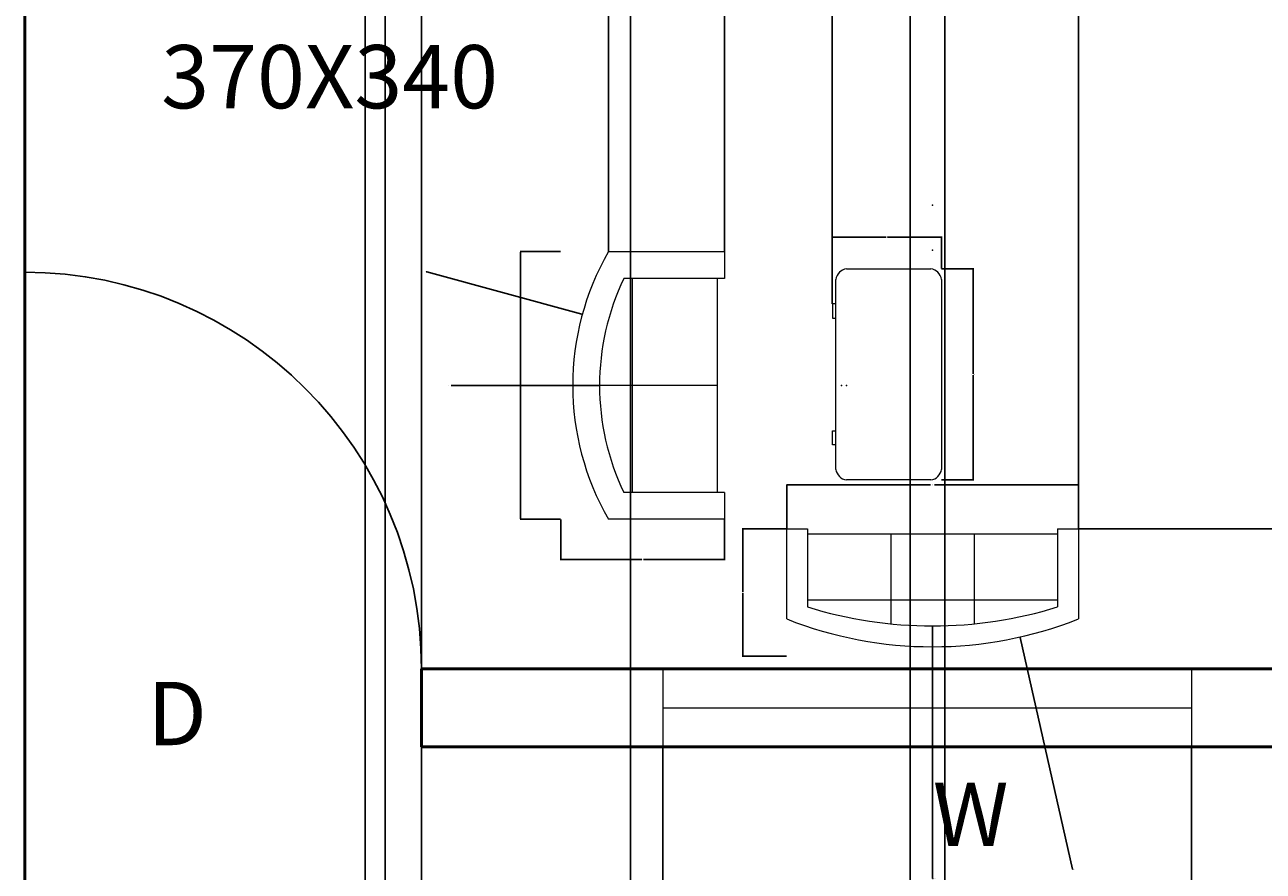
# Model space of a CAD drawing. Units: centimetres. Extents: x 2050 to 3144, y 831 to 2296.
# Tile 3 of 7: x 2553 to 2916, y 1152 to 1401. Entities that reach past the tile are written whole.
import ezdxf

# ---------------------------------------------------------------- set-up
doc = ezdxf.new("R2010")
doc.units = ezdxf.units.CM
for name, color, linetype, lineweight in [('A-ANNO-DIMS', 2, 'Continuous', 18), ('A-ANNO-TEXT', 7, 'Continuous', 18), ('A-AREA-IDEN', 7, 'Continuous', 25), ('A-DOOR', 3, 'Continuous', 25), ('A-FURN', 8, 'Continuous', 18), ('A-GLAZ', 4, 'Continuous', 18), ('A-WALL', 7, 'Continuous', 50)]:
    doc.layers.add(name, color=color, linetype=linetype, lineweight=lineweight)
doc.styles.get("Standard").update_dxf_attribs({"font": 'arial.ttf'})
doc.dimstyles.get("Standard").update_dxf_attribs({"dimtxt": 0.18, "dimasz": 0.18, "dimexe": 0.18, "dimexo": 0.0625, "dimgap": 0.09, "dimtad": 0, "dimtih": 1, "dimtoh": 1, "dimdec": 4, "dimzin": 0, "dimdsep": 46, "dimtxsty": 'Standard', "dimcen": 0.09, "dimadec": 0, "dimazin": 0, "dimtfac": 1, "dimtdec": 4, "dimtofl": 0, "dimtmove": 0, "dimatfit": 3, "dimfxl": 1, "dimtolj": 1, "dimtzin": 0, "dimarcsym": 0})

# ---------------------------------------------------------------- blocks, each defined once
blk = doc.blocks.new('Sofa - Roundback 7 ft.')
for p, q in [((-12.00002, -32.4421), (-12.00003, -6.5971)), ((11.99997, -32.4421), (11.99998, -6.5971)), ((-36.000027, -34), (-36.000027, -11.4696)), ((-35.999844, -13.3819), (35.9998, -13.3819)), ((35.99998, -34), (35.99998, -11.4696)), ((-36.000027, -32.4421), (35.99998, -32.4421))]:
    blk.add_line(p, q)
for points in [[(-36.000027, -34), (-42.000027, -34), (-42.000027, -8)], [(41.99998, -8), (41.99998, -34), (35.99998, -34)]]:
    blk.add_lwpolyline(points)
for centre, radius, start, end in [((0, -114.25), 114.25, 68.43141, 111.5686), ((-0.00001, -127.1968), 121.1968, 72.72033, 107.2797)]:
    blk.add_arc(centre, radius, start, end)
blk = doc.blocks.new('Sofa - Roundback Loveseat 5 ft.')
for p, q in [((0, -32.44198), (0, -5.99998)), ((-24, -33.99998), (-24, -11.46958)), ((-23.9998, -13.38178), (23.99986, -13.38178)), ((24.00004, -33.99998), (24.00004, -11.46958)), ((-24, -32.44198), (24.00004, -32.44198))]:
    blk.add_line(p, q)
for points in [[(-24, -33.99998), (-30, -33.99998), (-30, -7.99998)], [(30.00004, -7.99998), (30.00004, -33.99998), (24.00004, -33.99998)]]:
    blk.add_lwpolyline(points)
for centre, radius, start, end in [((0, -60.24998), 60.24998, 60.13715, 119.8628), ((0, -61.38438), 55.38444, 64.32083, 115.6792)]:
    blk.add_arc(centre, radius, start, end)
blk = doc.blocks.new('Desk - 30 x 60 in.')
for p, q in [((-26.999995, 0), (26.999995, 0)), ((-29.999995, -27), (-29.999995, -3)), ((29.999995, -3), (29.999995, -27)), ((26.999995, -30), (-26.999995, -30)), ((-20.000005, -30), (-20.000005, -31)), ((-20.000005, -31), (-16.000005, -31)), ((-16.000005, -31), (-16.000005, -30)), ((15.999995, -31), (15.999995, -30)), ((19.999995, -31), (15.999995, -31)), ((19.999995, -30), (19.999995, -31))]:
    blk.add_line(p, q)
for centre, start, end in [((-26.499995, -3.5), 98.1301, 171.8699), ((26.499995, -3.5), 8.130102, 81.8699), ((-26.499995, -26.5), 188.1301, 261.8699), ((26.499995, -26.5), 278.1301, 351.8699)]:
    blk.add_arc(centre, 3.535534, start, end)
blk = doc.blocks.new('*D21')
at = {"layer": 'A-ANNO-DIMS', "color": 0, "lineweight": -2, "transparency": 16777216}
for p, q in [((2776.49, 1253.11), (2776.49, 1266.08)), ((2776.67, 1265.9), (2818.72, 1265.9)), ((2861.97, 1265.9), (2819.91, 1265.9)), ((2862.15, 1253.11), (2862.15, 1266.08))]:
    blk.add_line(p, q, dxfattribs=at)
at = {"layer": 'A-ANNO-DIMS', "color": 0, "transparency": 16777216}
for points in [[(2776.67, 1265.93), (2776.67, 1265.87), (2776.49, 1265.9)], [(2861.97, 1265.93), (2861.97, 1265.87), (2862.15, 1265.9)]]:
    blk.add_solid(points, dxfattribs=at)
at = {"layer": 'Defpoints', "color": 0, "transparency": 16777216}
for p in [(2776.49, 1265.9), (2776.49, 1253.05), (2862.15, 1253.05)]:
    blk.add_point(p, dxfattribs=at)
at = {"layer": 'A-ANNO-DIMS', "color": 0, "transparency": 16777216, "insert": (2819.32, 1265.9), "char_height": 0.18, "attachment_point": 5}
blk.add_mtext('\\A1;SOFA 86', dxfattribs=at)
blk = doc.blocks.new('*D22')
at = {"layer": 'A-ANNO-DIMS', "color": 0, "lineweight": -2, "transparency": 16777216}
for p, q in [((2776.43, 1253.05), (2763.46, 1253.05)), ((2763.64, 1252.87), (2763.64, 1234.54)), ((2763.64, 1215.84), (2763.64, 1234.17)), ((2776.43, 1215.66), (2763.46, 1215.66))]:
    blk.add_line(p, q, dxfattribs=at)
at = {"layer": 'A-ANNO-DIMS', "color": 0, "transparency": 16777216}
for points in [[(2763.61, 1252.87), (2763.67, 1252.87), (2763.64, 1253.05)], [(2763.61, 1215.84), (2763.67, 1215.84), (2763.64, 1215.66)]]:
    blk.add_solid(points, dxfattribs=at)
at = {"layer": 'Defpoints', "color": 0, "transparency": 16777216}
for p in [(2776.49, 1253.05), (2763.64, 1215.66), (2776.49, 1215.66)]:
    blk.add_point(p, dxfattribs=at)
at = {"layer": 'A-ANNO-DIMS', "color": 0, "transparency": 16777216, "insert": (2763.64, 1234.36), "char_height": 0.18, "attachment_point": 5}
blk.add_mtext('\\A1;37', dxfattribs=at)
blk = doc.blocks.new('*D23')
at = {"layer": 'A-ANNO-DIMS', "color": 0, "lineweight": -2, "transparency": 16777216}
for p, q in [((2710.09, 1334.43), (2698.18, 1334.43)), ((2698.36, 1334.25), (2698.36, 1295.31)), ((2698.36, 1256), (2698.36, 1294.94)), ((2710.09, 1255.82), (2698.18, 1255.82))]:
    blk.add_line(p, q, dxfattribs=at)
at = {"layer": 'A-ANNO-DIMS', "color": 0, "transparency": 16777216}
for points in [[(2698.33, 1334.25), (2698.39, 1334.25), (2698.36, 1334.43)], [(2698.33, 1256), (2698.39, 1256), (2698.36, 1255.82)]]:
    blk.add_solid(points, dxfattribs=at)
at = {"layer": 'Defpoints', "color": 0, "transparency": 16777216}
for p in [(2698.36, 1334.43), (2710.16, 1334.43), (2710.16, 1255.82)]:
    blk.add_point(p, dxfattribs=at)
at = {"layer": 'A-ANNO-DIMS', "color": 0, "transparency": 16777216, "insert": (2698.36, 1295.12), "char_height": 0.18, "attachment_point": 5}
blk.add_mtext('\\A1;LOVESEAT 79', dxfattribs=at)
blk = doc.blocks.new('*D24')
at = {"layer": 'A-ANNO-DIMS', "color": 0, "lineweight": -2, "transparency": 16777216}
for p, q in [((2710.16, 1255.75), (2710.16, 1243.84)), ((2758.2, 1255.75), (2758.2, 1243.84)), ((2710.34, 1244.02), (2733.95, 1244.02)), ((2758.02, 1244.02), (2734.4, 1244.02))]:
    blk.add_line(p, q, dxfattribs=at)
at = {"layer": 'A-ANNO-DIMS', "color": 0, "transparency": 16777216}
for points in [[(2710.34, 1244.05), (2710.34, 1243.99), (2710.16, 1244.02)], [(2758.02, 1244.05), (2758.02, 1243.99), (2758.2, 1244.02)]]:
    blk.add_solid(points, dxfattribs=at)
at = {"layer": 'Defpoints', "color": 0, "transparency": 16777216}
for p in [(2710.16, 1255.82), (2758.2, 1255.82), (2710.16, 1244.02)]:
    blk.add_point(p, dxfattribs=at)
at = {"layer": 'A-ANNO-DIMS', "color": 0, "transparency": 16777216, "insert": (2734.18, 1244.02), "char_height": 0.18, "attachment_point": 5}
blk.add_mtext('\\A1;48', dxfattribs=at)
blk = doc.blocks.new('*D29')
at = {"layer": 'A-ANNO-DIMS', "color": 0, "lineweight": -2, "transparency": 16777216}
for p, q in [((2822, 1329.39), (2831.42, 1329.39)), ((2831.24, 1329.21), (2831.24, 1298.57)), ((2831.24, 1267.55), (2831.24, 1298.2)), ((2822, 1267.37), (2831.42, 1267.37))]:
    blk.add_line(p, q, dxfattribs=at)
at = {"layer": 'A-ANNO-DIMS', "color": 0, "transparency": 16777216}
for points in [[(2831.21, 1329.21), (2831.27, 1329.21), (2831.24, 1329.39)], [(2831.21, 1267.55), (2831.27, 1267.55), (2831.24, 1267.37)]]:
    blk.add_solid(points, dxfattribs=at)
at = {"layer": 'Defpoints', "color": 0, "transparency": 16777216}
for p in [(2821.94, 1329.39), (2821.94, 1267.37), (2831.24, 1267.37)]:
    blk.add_point(p, dxfattribs=at)
at = {"layer": 'A-ANNO-DIMS', "color": 0, "transparency": 16777216, "insert": (2831.24, 1298.38), "char_height": 0.18, "attachment_point": 5}
blk.add_mtext('\\A1;DESK 62', dxfattribs=at)
blk = doc.blocks.new('*D30')
at = {"layer": 'A-ANNO-DIMS', "color": 0, "lineweight": -2, "transparency": 16777216}
for p, q in [((2789.89, 1329.46), (2789.89, 1338.88)), ((2790.07, 1338.7), (2805.7, 1338.7)), ((2821.76, 1338.7), (2806.14, 1338.7)), ((2821.94, 1329.46), (2821.94, 1338.88))]:
    blk.add_line(p, q, dxfattribs=at)
at = {"layer": 'A-ANNO-DIMS', "color": 0, "transparency": 16777216}
for points in [[(2790.07, 1338.73), (2790.07, 1338.67), (2789.89, 1338.7)], [(2821.76, 1338.73), (2821.76, 1338.67), (2821.94, 1338.7)]]:
    blk.add_solid(points, dxfattribs=at)
at = {"layer": 'Defpoints', "color": 0, "transparency": 16777216}
for p in [(2821.94, 1338.7), (2789.89, 1329.39), (2821.94, 1329.39)]:
    blk.add_point(p, dxfattribs=at)
at = {"layer": 'A-ANNO-DIMS', "color": 0, "transparency": 16777216, "insert": (2805.92, 1338.7), "char_height": 0.18, "attachment_point": 5}
blk.add_mtext('\\A1;32', dxfattribs=at)
blk = doc.blocks.new('*D48')
at = {"layer": 'A-ANNO-DIMS', "color": 0, "lineweight": -2, "transparency": 16777216}
for p, q in [((2552.73, 1211.94), (2552.73, 2154.53)), ((2552.91, 2154.35), (2610.59, 2154.35)), ((2669.05, 2154.35), (2611.37, 2154.35)), ((2669.23, 1211.94), (2669.23, 2154.53))]:
    blk.add_line(p, q, dxfattribs=at)
at = {"layer": 'A-ANNO-DIMS', "color": 0, "transparency": 16777216}
for points in [[(2552.91, 2154.38), (2552.91, 2154.32), (2552.73, 2154.35)], [(2669.05, 2154.38), (2669.05, 2154.32), (2669.23, 2154.35)]]:
    blk.add_solid(points, dxfattribs=at)
at = {"layer": 'Defpoints', "color": 0, "transparency": 16777216}
for p in [(2669.23, 2154.35), (2552.73, 1211.87), (2669.23, 1211.87)]:
    blk.add_point(p, dxfattribs=at)
at = {"layer": 'A-ANNO-DIMS', "color": 0, "transparency": 16777216, "insert": (2610.98, 2154.35), "char_height": 0.18, "attachment_point": 5}
blk.add_mtext('\\A1;116.5', dxfattribs=at)
blk = doc.blocks.new('*D49')
at = {"layer": 'A-ANNO-DIMS', "color": 0, "lineweight": -2, "transparency": 16777216}
for p, q in [((2669.23, 1188.95), (2669.23, 1009.53)), ((2740.09, 1188.95), (2740.09, 1009.53)), ((2669.41, 1009.71), (2704.27, 1009.71)), ((2739.91, 1009.71), (2705.05, 1009.71))]:
    blk.add_line(p, q, dxfattribs=at)
at = {"layer": 'A-ANNO-DIMS', "color": 0, "transparency": 16777216}
for points in [[(2669.41, 1009.74), (2669.41, 1009.68), (2669.23, 1009.71)], [(2739.91, 1009.74), (2739.91, 1009.68), (2740.09, 1009.71)]]:
    blk.add_solid(points, dxfattribs=at)
at = {"layer": 'Defpoints', "color": 0, "transparency": 16777216}
for p in [(2669.23, 1189.01), (2740.09, 1189.01), (2740.09, 1009.71)]:
    blk.add_point(p, dxfattribs=at)
at = {"layer": 'A-ANNO-DIMS', "color": 0, "transparency": 16777216, "insert": (2704.66, 1009.71), "char_height": 0.18, "attachment_point": 5}
blk.add_mtext('\\A1;70.86', dxfattribs=at)
blk = doc.blocks.new('*D50')
at = {"layer": 'A-ANNO-DIMS', "color": 0, "lineweight": -2, "transparency": 16777216}
for p, q in [((2740.09, 1188.95), (2740.09, 1009.53)), ((2895.36, 1188.95), (2895.36, 1009.53)), ((2740.27, 1009.71), (2817.27, 1009.71)), ((2895.18, 1009.71), (2818.18, 1009.71))]:
    blk.add_line(p, q, dxfattribs=at)
at = {"layer": 'A-ANNO-DIMS', "color": 0, "transparency": 16777216}
for points in [[(2740.27, 1009.74), (2740.27, 1009.68), (2740.09, 1009.71)], [(2895.18, 1009.74), (2895.18, 1009.68), (2895.36, 1009.71)]]:
    blk.add_solid(points, dxfattribs=at)
at = {"layer": 'Defpoints', "color": 0, "transparency": 16777216}
for p in [(2740.09, 1189.01), (2895.36, 1189.01), (2895.36, 1009.71)]:
    blk.add_point(p, dxfattribs=at)
at = {"layer": 'A-ANNO-DIMS', "color": 0, "transparency": 16777216, "insert": (2817.72, 1009.71), "char_height": 0.18, "attachment_point": 5}
blk.add_mtext('\\A1;155.27', dxfattribs=at)
blk = doc.blocks.new('*D59')
at = {"layer": 'A-ANNO-DIMS', "color": 0, "lineweight": -2, "transparency": 16777216}
for p, q in [((2862.15, 1253.11), (2862.15, 2154.53)), ((2862.33, 2154.35), (2907.04, 2154.35)), ((2952.55, 2154.35), (2907.83, 2154.35)), ((2952.73, 1211.94), (2952.73, 2154.53))]:
    blk.add_line(p, q, dxfattribs=at)
at = {"layer": 'A-ANNO-DIMS', "color": 0, "transparency": 16777216}
for points in [[(2862.33, 2154.38), (2862.33, 2154.32), (2862.15, 2154.35)], [(2952.55, 2154.38), (2952.55, 2154.32), (2952.73, 2154.35)]]:
    blk.add_solid(points, dxfattribs=at)
at = {"layer": 'Defpoints', "color": 0, "transparency": 16777216}
for p in [(2952.73, 2154.35), (2862.15, 1253.05), (2952.73, 1211.87)]:
    blk.add_point(p, dxfattribs=at)
at = {"layer": 'A-ANNO-DIMS', "color": 0, "transparency": 16777216, "insert": (2907.44, 2154.35), "char_height": 0.18, "attachment_point": 5}
blk.add_mtext('\\A1;90.58', dxfattribs=at)
blk = doc.blocks.new('*D60')
at = {"layer": 'A-ANNO-DIMS', "color": 0, "lineweight": -2, "transparency": 16777216}
for p, q in [((2862.21, 1253.05), (3042.37, 1253.05)), ((3042.19, 1252.87), (3042.19, 1232.65)), ((3042.19, 1212.05), (3042.19, 1232.28)), ((2895.42, 1211.87), (3042.37, 1211.87))]:
    blk.add_line(p, q, dxfattribs=at)
at = {"layer": 'A-ANNO-DIMS', "color": 0, "transparency": 16777216}
for points in [[(3042.16, 1252.87), (3042.22, 1252.87), (3042.19, 1253.05)], [(3042.16, 1212.05), (3042.22, 1212.05), (3042.19, 1211.87)]]:
    blk.add_solid(points, dxfattribs=at)
at = {"layer": 'Defpoints', "color": 0, "transparency": 16777216}
for p in [(2862.15, 1253.05), (2895.36, 1211.87), (3042.19, 1211.87)]:
    blk.add_point(p, dxfattribs=at)
at = {"layer": 'A-ANNO-DIMS', "color": 0, "transparency": 16777216, "insert": (3042.19, 1232.46), "char_height": 0.18, "attachment_point": 5}
blk.add_mtext('\\A1;41.18', dxfattribs=at)
blk = doc.blocks.new('*D61')
at = {"layer": 'A-ANNO-DIMS', "color": 0, "lineweight": -2, "transparency": 16777216}
for p, q in [((2552.73, 1328.44), (2552.73, 2154.53)), ((2552.91, 2154.35), (2638.04, 2154.35)), ((2723.95, 2154.35), (2638.81, 2154.35)), ((2724.13, 1334.5), (2724.13, 2154.53))]:
    blk.add_line(p, q, dxfattribs=at)
at = {"layer": 'A-ANNO-DIMS', "color": 0, "transparency": 16777216}
for points in [[(2552.91, 2154.38), (2552.91, 2154.32), (2552.73, 2154.35)], [(2723.95, 2154.38), (2723.95, 2154.32), (2724.13, 2154.35)]]:
    blk.add_solid(points, dxfattribs=at)
at = {"layer": 'Defpoints', "color": 0, "transparency": 16777216}
for p in [(2724.13, 2154.35), (2724.13, 1334.43), (2552.73, 1328.38)]:
    blk.add_point(p, dxfattribs=at)
at = {"layer": 'A-ANNO-DIMS', "color": 0, "transparency": 16777216, "insert": (2638.43, 2154.35), "char_height": 0.18, "attachment_point": 5}
blk.add_mtext('\\A1;171.4', dxfattribs=at)
blk = doc.blocks.new('*D62')
at = {"layer": 'A-ANNO-DIMS', "color": 0, "lineweight": -2, "transparency": 16777216}
for p, q in [((2758.2, 1334.5), (2758.2, 2154.53)), ((2758.38, 2154.35), (2773.58, 2154.35)), ((2789.71, 2154.35), (2774.51, 2154.35)), ((2789.89, 1319.12), (2789.89, 2154.53))]:
    blk.add_line(p, q, dxfattribs=at)
at = {"layer": 'A-ANNO-DIMS', "color": 0, "transparency": 16777216}
for points in [[(2758.38, 2154.38), (2758.38, 2154.32), (2758.2, 2154.35)], [(2789.71, 2154.38), (2789.71, 2154.32), (2789.89, 2154.35)]]:
    blk.add_solid(points, dxfattribs=at)
at = {"layer": 'Defpoints', "color": 0, "transparency": 16777216}
for p in [(2789.89, 2154.35), (2758.2, 1334.43), (2789.89, 1319.06)]:
    blk.add_point(p, dxfattribs=at)
at = {"layer": 'A-ANNO-DIMS', "color": 0, "transparency": 16777216, "insert": (2774.05, 2154.35), "char_height": 0.18, "attachment_point": 5}
blk.add_mtext('\\A1;31.696', dxfattribs=at)
blk = doc.blocks.new('*D65')
at = {"layer": 'A-ANNO-DIMS', "color": 0, "lineweight": -2, "transparency": 16777216}
for p, q in [((2812.73, 1924.83), (2812.73, 1009.53)), ((2822.89, 1914.67), (2822.89, 1009.53)), ((2812.91, 1009.71), (2817.42, 1009.71)), ((2822.71, 1009.71), (2818.19, 1009.71))]:
    blk.add_line(p, q, dxfattribs=at)
at = {"layer": 'A-ANNO-DIMS', "color": 0, "transparency": 16777216}
for points in [[(2812.91, 1009.74), (2812.91, 1009.68), (2812.73, 1009.71)], [(2822.71, 1009.74), (2822.71, 1009.68), (2822.89, 1009.71)]]:
    blk.add_solid(points, dxfattribs=at)
at = {"layer": 'Defpoints', "color": 0, "transparency": 16777216}
for p in [(2812.73, 1924.89), (2822.89, 1914.73), (2822.89, 1009.71)]:
    blk.add_point(p, dxfattribs=at)
at = {"layer": 'A-ANNO-DIMS', "color": 0, "transparency": 16777216, "insert": (2817.81, 1009.71), "char_height": 0.18, "attachment_point": 5}
blk.add_mtext('\\A1;10.16', dxfattribs=at)
blk = doc.blocks.new('*D68')
at = {"layer": 'A-ANNO-DIMS', "color": 0, "lineweight": -2, "transparency": 16777216}
for p, q in [((2652.73, 1914.67), (2652.73, 1009.53)), ((2730.58, 1841.3), (2730.58, 1009.53)), ((2652.91, 1009.71), (2691.26, 1009.71)), ((2730.4, 1009.71), (2692.05, 1009.71))]:
    blk.add_line(p, q, dxfattribs=at)
at = {"layer": 'A-ANNO-DIMS', "color": 0, "transparency": 16777216}
for points in [[(2652.91, 1009.74), (2652.91, 1009.68), (2652.73, 1009.71)], [(2730.4, 1009.74), (2730.4, 1009.68), (2730.58, 1009.71)]]:
    blk.add_solid(points, dxfattribs=at)
at = {"layer": 'Defpoints', "color": 0, "transparency": 16777216}
for p in [(2652.73, 1914.73), (2730.58, 1841.36), (2730.58, 1009.71)]:
    blk.add_point(p, dxfattribs=at)
at = {"layer": 'A-ANNO-DIMS', "color": 0, "transparency": 16777216, "insert": (2691.65, 1009.71), "char_height": 0.18, "attachment_point": 5}
blk.add_mtext('\\A1;77.85', dxfattribs=at)
blk = doc.blocks.new('*D73')
at = {"layer": 'A-ANNO-DIMS', "color": 0, "lineweight": -2, "transparency": 16777216}
for p, q in [((2658.57, 1971.45), (2658.57, 1009.53)), ((2652.73, 1924.83), (2652.73, 1009.53)), ((2652.91, 1009.71), (2655.26, 1009.71)), ((2658.39, 1009.71), (2656.04, 1009.71))]:
    blk.add_line(p, q, dxfattribs=at)
at = {"layer": 'A-ANNO-DIMS', "color": 0, "transparency": 16777216}
for points in [[(2652.91, 1009.74), (2652.91, 1009.68), (2652.73, 1009.71)], [(2658.39, 1009.74), (2658.39, 1009.68), (2658.57, 1009.71)]]:
    blk.add_solid(points, dxfattribs=at)
at = {"layer": 'Defpoints', "color": 0, "transparency": 16777216}
for p in [(2658.57, 1971.51), (2652.73, 1924.89), (2658.57, 1009.71)]:
    blk.add_point(p, dxfattribs=at)
at = {"layer": 'A-ANNO-DIMS', "color": 0, "transparency": 16777216, "insert": (2655.65, 1009.71), "char_height": 0.18, "attachment_point": 5}
blk.add_mtext('\\A1;5.847', dxfattribs=at)
blk = doc.blocks.new('*D74')
at = {"layer": 'A-ANNO-DIMS', "color": 0, "lineweight": -2, "transparency": 16777216}
for p, q in [((2952.73, 2064.83), (2952.73, 1009.53)), ((2822.89, 2004.16), (2822.89, 1009.53)), ((2823.07, 1009.71), (2887.35, 1009.71)), ((2952.55, 1009.71), (2888.26, 1009.71))]:
    blk.add_line(p, q, dxfattribs=at)
at = {"layer": 'A-ANNO-DIMS', "color": 0, "transparency": 16777216}
for points in [[(2823.07, 1009.74), (2823.07, 1009.68), (2822.89, 1009.71)], [(2952.55, 1009.74), (2952.55, 1009.68), (2952.73, 1009.71)]]:
    blk.add_solid(points, dxfattribs=at)
at = {"layer": 'Defpoints', "color": 0, "transparency": 16777216}
for p in [(2952.73, 2064.89), (2822.89, 2004.22), (2952.73, 1009.71)]:
    blk.add_point(p, dxfattribs=at)
at = {"layer": 'A-ANNO-DIMS', "color": 0, "transparency": 16777216, "insert": (2887.81, 1009.71), "char_height": 0.18, "attachment_point": 5}
blk.add_mtext('\\A1;129.84', dxfattribs=at)
blk = doc.blocks.new('*D77')
at = {"layer": 'A-ANNO-DIMS', "color": 0, "lineweight": -2, "transparency": 16777216}
for p, q in [((2819.23, 1348.09), (2819.41, 1348.09)), ((2819.32, 1348), (2819.32, 1348.18)), ((2819.32, 1150.35), (2819.32, 1224.32)), ((2819.5, 1150.35), (2819.32, 1150.35))]:
    blk.add_line(p, q, dxfattribs=at)
at = {"layer": 'A-ANNO-DIMS', "color": 0, "transparency": 16777216}
blk.add_solid([(2819.35, 1224.32), (2819.29, 1224.32), (2819.32, 1224.5)], dxfattribs=at)
at = {"layer": 'Defpoints', "color": 0, "transparency": 16777216}
for p in [(2819.32, 1348.09), (2819.32, 1224.5)]:
    blk.add_point(p, dxfattribs=at)
at = {"layer": 'A-ANNO-DIMS', "color": 0, "transparency": 16777216, "insert": (2820.05, 1150.35), "char_height": 0.18, "attachment_point": 5}
blk.add_mtext('\\A1;R123.59', dxfattribs=at)
blk = doc.blocks.new('*D78')
at = {"layer": 'A-ANNO-DIMS', "color": 0, "lineweight": -2, "transparency": 16777216}
for p, q in [((2819.23, 1334.88), (2819.41, 1334.88)), ((2819.32, 1334.79), (2819.32, 1334.97)), ((2860.41, 1153.07), (2845.04, 1221.07)), ((2860.59, 1153.07), (2860.41, 1153.07))]:
    blk.add_line(p, q, dxfattribs=at)
at = {"layer": 'A-ANNO-DIMS', "color": 0, "transparency": 16777216}
blk.add_solid([(2845.07, 1221.08), (2845.01, 1221.07), (2845, 1221.25)], dxfattribs=at)
at = {"layer": 'Defpoints', "color": 0, "transparency": 16777216}
for p in [(2819.32, 1334.88), (2845, 1221.25)]:
    blk.add_point(p, dxfattribs=at)
at = {"layer": 'A-ANNO-DIMS', "color": 0, "transparency": 16777216, "insert": (2861.07, 1153.07), "char_height": 0.18, "attachment_point": 5}
blk.add_mtext('\\A1;R116.5', dxfattribs=at)
blk = doc.blocks.new('*D79')
at = {"layer": 'A-ANNO-DIMS', "color": 0, "lineweight": -2, "transparency": 16777216}
for p, q in [((2670.6, 1328.54), (2670.78, 1328.54)), ((2670.78, 1328.54), (2716.29, 1316.06)), ((2792.5, 1295.12), (2792.68, 1295.12)), ((2792.59, 1295.03), (2792.59, 1295.21))]:
    blk.add_line(p, q, dxfattribs=at)
at = {"layer": 'A-ANNO-DIMS', "color": 0, "transparency": 16777216}
blk.add_solid([(2716.3, 1316.09), (2716.28, 1316.03), (2716.46, 1316.01)], dxfattribs=at)
at = {"layer": 'Defpoints', "color": 0, "transparency": 16777216}
for p in [(2716.46, 1316.01), (2792.59, 1295.12)]:
    blk.add_point(p, dxfattribs=at)
at = {"layer": 'A-ANNO-DIMS', "color": 0, "transparency": 16777216, "insert": (2670.12, 1328.54), "char_height": 0.18, "attachment_point": 5}
blk.add_mtext('\\A1;R78.94', dxfattribs=at)
blk = doc.blocks.new('*D80')
at = {"layer": 'A-ANNO-DIMS', "color": 0, "lineweight": -2, "transparency": 16777216}
for p, q in [((2677.97, 1295.12), (2721.33, 1295.12)), ((2793.99, 1295.12), (2794.17, 1295.12)), ((2794.08, 1295.03), (2794.08, 1295.21))]:
    blk.add_line(p, q, dxfattribs=at)
at = {"layer": 'A-ANNO-DIMS', "color": 0, "transparency": 16777216}
blk.add_solid([(2721.33, 1295.16), (2721.33, 1295.1), (2721.51, 1295.12)], dxfattribs=at)
at = {"layer": 'Defpoints', "color": 0, "transparency": 16777216}
for p in [(2721.51, 1295.12), (2794.08, 1295.12)]:
    blk.add_point(p, dxfattribs=at)
at = {"layer": 'A-ANNO-DIMS', "color": 0, "transparency": 16777216, "insert": (2677.49, 1295.12), "char_height": 0.18, "attachment_point": 5}
blk.add_mtext('\\A1;R72.57', dxfattribs=at)

msp = doc.modelspace()

# ---------------------------------------------------------------- linework, layer by layer
at = {"layer": 'A-DOOR'}
msp.add_line((2552.7265, 1211.8748), (2552.7265, 1338.3548), dxfattribs=at)
msp.add_arc((2552.7265, 1211.8748), 116.5053, 0, 90, dxfattribs=at)
at = {"layer": 'A-GLAZ'}
for p, q in [((2740.0885, 1211.8748), (2740.0885, 1189.0148)), ((2895.3598, 1211.8748), (2895.3598, 1189.0148)), ((2740.0885, 1200.4448), (2895.3598, 1200.4448))]:
    msp.add_line(p, q, dxfattribs=at)
at = {"layer": 'A-WALL'}
for p, q in [((2552.7265, 1076.3148), (2552.7265, 1442.0348)), ((2952.7265, 1211.8748), (2669.2319, 1211.8748)), ((2669.2319, 1211.8748), (2669.2319, 1189.0148)), ((2975.5865, 1189.0148), (2669.2319, 1189.0148))]:
    msp.add_line(p, q, dxfattribs=at)

# ---------------------------------------------------------------- block references
at = {"layer": 'A-FURN'}
for name, p, xscale, yscale, zscale, rotation in [('Sofa - Roundback Loveseat 5 ft.', (2713.6496, 1295.1248), 1.310271314110985, 1.310271314110985, 1.310271314110985, 90), ('Desk - 30 x 60 in.', (2821.9397, 1298.3823), 1.033716000935604, 1.033716000935604, 1.033716000935604, 270), ('Sofa - Roundback 7 ft.', (2819.3175, 1218.3814), 1.019710447399378, 1.019710447399378, 1.019710447399378, 180)]:
    msp.add_blockref(name, p, dxfattribs=dict(at, xscale=xscale, yscale=yscale, zscale=zscale, rotation=rotation))

# ---------------------------------------------------------------- texts
at = {"layer": 'A-ANNO-TEXT'}
for s, p in [('D', (2588.744, 1189.4801)), ('W', (2819.3819, 1159.8805))]:
    msp.add_text(s, height=18.5959, dxfattribs=at).set_placement(p)
at = {"layer": 'A-AREA-IDEN'}
msp.add_text('370X340', height=18.57938, dxfattribs=at).set_placement((2592.7975, 1376.5242))

# ---------------------------------------------------------------- dimensions: what is measured, and where the dimension line sits
at = {"layer": 'A-ANNO-DIMS'}
for base, p1, p2, override, picture, middle in [((2669.2319, 2154.3548), (2552.7265, 1211.8748), (2669.2319, 1211.8748), {"dimdec": 1, "dimlfac": 1, "dimrnd": 0, "dimzin": 0, "dimdsep": 46, "dimlunit": 2}, '*D48', (2610.9792, 2154.3548)), ((2724.1318, 2154.3548), (2552.7265, 1328.3801), (2724.1318, 1334.433), {"dimdec": 1, "dimlfac": 1, "dimrnd": 0, "dimzin": 0, "dimdsep": 46, "dimlunit": 2}, '*D61', (2638.4292, 2154.3548)), ((2789.8945, 2154.3548), (2758.1988, 1334.433), (2789.8945, 1319.0567), {"dimdec": 3, "dimlfac": 1, "dimrnd": 0, "dimzin": 0, "dimdsep": 46, "dimlunit": 2}, '*D62', (2774.0467, 2154.3548)), ((2952.7265, 2154.3548), (2862.1454, 1253.0515), (2952.7265, 1211.8748), {"dimdec": 2, "dimlfac": 1, "dimrnd": 0, "dimzin": 0, "dimdsep": 46, "dimlunit": 2}, '*D59', (2907.436, 2154.3548)), ((2952.7265, 1009.7148), (2822.8865, 2004.2202), (2952.7265, 2064.8948), {"dimdec": 2, "dimlfac": 1, "dimrnd": 0, "dimzin": 0, "dimdsep": 46, "dimlunit": 2}, '*D74', (2887.8065, 1009.7148)), ((2658.5737, 1009.7148), (2652.7265, 1924.8948), (2658.5737, 1971.5118), {"dimdec": 3, "dimlfac": 1, "dimrnd": 0, "dimzin": 0, "dimdsep": 46, "dimlunit": 2}, '*D73', (2655.6501, 1009.7148)), ((2822.8865, 1009.7148), (2812.7265, 1924.8948), (2822.8865, 1914.7348), {"dimdec": 2, "dimlfac": 1, "dimrnd": 0, "dimzin": 0, "dimdsep": 46, "dimlunit": 2}, '*D65', (2817.8065, 1009.7148)), ((2730.579, 1009.7148), (2652.7265, 1914.7348), (2730.579, 1841.3577), {"dimdec": 2, "dimlfac": 1, "dimrnd": 0, "dimzin": 0, "dimdsep": 46, "dimlunit": 2}, '*D68', (2691.6528, 1009.7148)), ((2821.9397, 1338.6973), (2789.8945, 1329.3938), (2821.9397, 1329.3938), {"dimdec": 0, "dimlfac": 1, "dimrnd": 0, "dimzin": 0, "dimdsep": 46, "dimlunit": 2}, '*D30', (2805.9171, 1338.6973)), ((2740.0885, 1009.7148), (2669.2319, 1189.0148), (2740.0885, 1189.0148), {"dimdec": 2, "dimlfac": 1, "dimrnd": 0, "dimzin": 0, "dimdsep": 46, "dimlunit": 2}, '*D49', (2704.6602, 1009.7148)), ((2895.3598, 1009.7148), (2740.0885, 1189.0148), (2895.3598, 1189.0148), {"dimdec": 2, "dimlfac": 1, "dimrnd": 0, "dimzin": 0, "dimdsep": 46, "dimlunit": 2}, '*D50', (2817.7241, 1009.7148))]:
    dim = msp.add_linear_dim(base=base, p1=p1, p2=p2, dimstyle='Standard', override=override, dxfattribs=at)
    dim.commit()
    dim.dimension.update_dxf_attribs({"geometry": picture, "text_midpoint": middle})
for center, mpoint, override, picture, middle in [((2819.3175, 1348.0853), (2819.318, 1224.4996), {"dimdec": 2, "dimlfac": 1, "dimrnd": 0, "dimzin": 0, "dimdsep": 46, "dimlunit": 2}, '*D77', (2820.0482, 1150.3483)), ((2819.3175, 1334.8833), (2845.0005, 1221.2476), {"dimdec": 1, "dimlfac": 1, "dimrnd": 0, "dimzin": 0, "dimdsep": 46, "dimlunit": 2}, '*D78', (2861.0709, 1153.0661)), ((2792.5935, 1295.1248), (2716.4625, 1316.0103), {"dimdec": 2, "dimlfac": 1, "dimrnd": 0, "dimzin": 0, "dimdsep": 46, "dimlunit": 2}, '*D79', (2670.1244, 1328.5416)), ((2794.0798, 1295.1248), (2721.5112, 1295.125), {"dimdec": 2, "dimlfac": 1, "dimrnd": 0, "dimzin": 0, "dimdsep": 46, "dimlunit": 2}, '*D80', (2677.97, 1295.1251))]:
    dim = msp.add_radius_dim(center=center, mpoint=mpoint, dimstyle='Standard', override=override, dxfattribs=at)
    dim.commit()
    dim.dimension.update_dxf_attribs({"geometry": picture, "text_midpoint": middle, "dimtype": 164})
for base, p1, p2, angle, text, picture, middle in [((2698.3631, 1334.433), (2710.1556, 1255.8167), (2710.1556, 1334.433), 90, 'LOVESEAT <>', '*D23', (2698.3631, 1295.1249)), ((2831.2432, 1267.3709), (2821.9397, 1329.3938), (2821.9397, 1267.3709), 270, 'DESK <>', '*D29', (2831.2432, 1298.3823)), ((2776.4897, 1265.8999), (2862.1454, 1253.0515), (2776.4897, 1253.0515), 180, 'SOFA <>', '*D21', (2819.3175, 1265.8999))]:
    dim = msp.add_linear_dim(base=base, p1=p1, p2=p2, angle=angle, text=text, dimstyle='Standard', override={"dimdec": 0, "dimlfac": 1, "dimrnd": 0, "dimzin": 0, "dimdsep": 46, "dimlunit": 2}, dxfattribs=at)
    dim.commit()
    dim.dimension.update_dxf_attribs({"geometry": picture, "text_midpoint": middle})
for base, p1, p2, angle, override, picture, middle in [((2710.1556, 1244.0242), (2758.1988, 1255.8167), (2710.1556, 1255.8167), 180, {"dimdec": 0, "dimlfac": 1, "dimrnd": 0, "dimzin": 0, "dimdsep": 46, "dimlunit": 2}, '*D24', (2734.1772, 1244.0242)), ((2763.6413, 1215.6622), (2776.4897, 1253.0515), (2776.4897, 1215.6622), 270, {"dimdec": 0, "dimlfac": 1, "dimrnd": 0, "dimzin": 0, "dimdsep": 46, "dimlunit": 2}, '*D22', (2763.6413, 1234.3568)), ((3042.1865, 1211.8748), (2862.1454, 1253.0515), (2895.3598, 1211.8748), 90, {"dimdec": 2, "dimlfac": 1, "dimrnd": 0, "dimzin": 0, "dimdsep": 46, "dimlunit": 2}, '*D60', (3042.1865, 1232.4632))]:
    dim = msp.add_linear_dim(base=base, p1=p1, p2=p2, angle=angle, dimstyle='Standard', override=override, dxfattribs=at)
    dim.commit()
    dim.dimension.update_dxf_attribs({"geometry": picture, "text_midpoint": middle})

doc.saveas('drawing.dxf')
